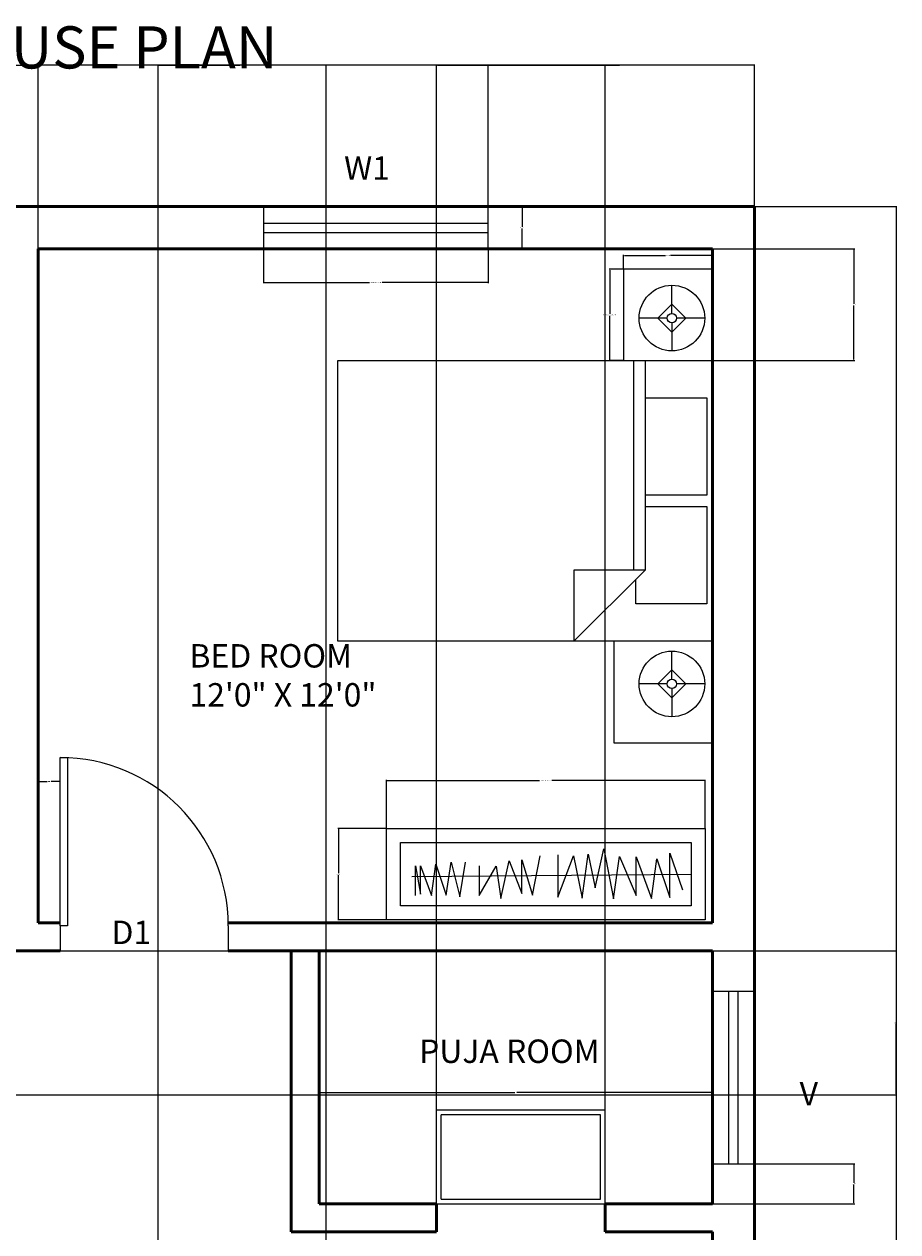
# Model space of a CAD drawing. Units: inches. Extents: x 437 to 811, y 2074 to 2699.
# Tile 4 of 4: x 624 to 811, y 2441 to 2699. Entities that reach past the tile are written whole.
import ezdxf

# ---------------------------------------------------------------- set-up
doc = ezdxf.new("R2010")
doc.units = ezdxf.units.IN
for name, color, linetype, lineweight in [('A-ANNO-DIMS', 2, 'Continuous', 18), ('A-ANNO-TEXT', 7, 'Continuous', 18), ('A-ANNO-TTLB', 7, 'Continuous', 35), ('A-AREA-IDEN', 7, 'Continuous', 25), ('A-DOOR', 4, 'Continuous', 25), ('A-FLOR-CASE', 9, 'Continuous', 25), ('A-FURN', 8, 'Continuous', 18), ('A-GLAZ', 4, 'Continuous', 18), ('A-WALL', 7, 'Continuous', 50)]:
    doc.layers.add(name, color=color, linetype=linetype, lineweight=lineweight)
doc.styles.get("Standard").update_dxf_attribs({"font": 'arial.ttf'})
doc.dimstyles.get("Standard").update_dxf_attribs({"dimtxt": 0.18, "dimasz": 0.18, "dimexe": 0.18, "dimexo": 0.0625, "dimgap": 0.09, "dimtad": 0, "dimtih": 1, "dimtoh": 1, "dimdec": 4, "dimzin": 0, "dimdsep": 46, "dimtxsty": 'Standard', "dimcen": 0.09, "dimadec": 0, "dimazin": 0, "dimtfac": 1, "dimtdec": 4, "dimtofl": 0, "dimtmove": 0, "dimatfit": 3, "dimfxl": 1, "dimtolj": 1, "dimtzin": 0, "dimarcsym": 0})

# ---------------------------------------------------------------- blocks, each defined once
blk = doc.blocks.new('Bed - Queen')
for p, q in [((0, -80.00003), (0, 0)), ((0, 0), (59.99999, 0)), ((59.99999, 0), (59.99999, -80.00003)), ((7.99999, -1.2), (28.79998, -1.2)), ((7.99999, -14.4), (7.99999, -1.2)), ((28.79998, -1.2), (28.79998, -14.4)), ((31.19999, -1.2), (51.99999, -1.2)), ((31.19999, -14.4), (31.19999, -1.2)), ((51.99999, -1.2), (51.99999, -16.4)), ((0, -14.4), (44.8, -14.4)), ((59.99999, -29.6), (44.8, -14.4)), ((44.8, -14.4), (44.8, -29.6)), ((44.8, -16.8), (0, -16.8)), ((51.99999, -16.4), (46.79936, -16.4)), ((44.8, -29.6), (59.99999, -29.6)), ((59.99999, -80.00003), (0, -80.00003))]:
    blk.add_line(p, q)
blk = doc.blocks.new('Lamp - Table')
for p, q in [((0, 7), (0, 1)), ((0, 3), (-3, 0)), ((3, 0), (0, 3)), ((-1, 0), (-7, 0)), ((-3, 0), (0, -3)), ((0, -3), (3, 0)), ((1, 0), (7, 0)), ((0, -1), (0, -7))]:
    blk.add_line(p, q)
for radius in [7, 1]:
    blk.add_circle((0, 0), radius)
blk = doc.blocks.new('*U10')
for p, q in [((0, 0), (0, -6)), ((40, 0), (40, -6))]:
    blk.add_line(p, q)
blk.add_lwpolyline([(0, 0), (0, 40), (1.75, 40), (1.75, 0)], close=True)
blk.add_arc((0, 0), 40, 0, 90)
blk = doc.blocks.new('WIN-W1-48IN')
for p, q in [((0, 5.5), (48, 5.5)), ((0, 3.5), (48, 3.5))]:
    blk.add_line(p, q)
blk.add_lwpolyline([(0, 0), (48, 0), (48, 9), (0, 9)], close=True)
blk = doc.blocks.new('VENT-V')
for p, q in [((9, 36.83), (0, 36.83)), ((0, 36.83), (0, 0)), ((3.5, 0), (3.5, 36.83)), ((5.5, 0), (5.5, 36.83)), ((9, 0), (9, 36.83)), ((0, 0), (9, 0))]:
    blk.add_line(p, q)
blk = doc.blocks.new('WARDROBE-BEDROOM')
for p, q in [((31.2, 5.25), (32.85, 13.72)), ((36.63, 13.91), (36.63, 4.86)), ((36.63, 4.86), (39.94, 13.72)), ((39.94, 13.72), (41.79, 4.67)), ((41.79, 4.67), (43.13, 14.04)), ((43.13, 14.04), (44.6, 6.84)), ((44.6, 6.84), (46.44, 15.19)), ((46.44, 15.19), (48.48, 4.48)), ((48.48, 4.48), (49.82, 13.53)), ((49.82, 13.53), (53.33, 5.18)), ((53.33, 5.18), (53.33, 13.47)), ((53.33, 13.47), (56.64, 4.54)), ((56.64, 4.54), (57.73, 13.02)), ((57.73, 13.02), (60.53, 4.8)), ((60.53, 4.8), (60.53, 14.29)), ((60.53, 14.29), (63.21, 6.39)), ((6.24, 5.24), (6.24, 11.53)), ((6.24, 11.53), (7.31, 5.48)), ((7.31, 5.48), (7.31, 11.54)), ((7.31, 11.54), (9.63, 5.2)), ((9.63, 5.2), (10.54, 11.9)), ((10.54, 11.9), (12.78, 5.28)), ((12.78, 5.28), (13.81, 12.34)), ((13.81, 12.34), (15.69, 4.96)), ((15.69, 4.96), (16.88, 12.37)), ((19.79, 11.56), (19.79, 5.18)), ((19.79, 5.18), (23.42, 11.48)), ((23.42, 11.48), (24.44, 4.55)), ((24.44, 4.55), (26.22, 12.64)), ((26.22, 12.64), (28.9, 5.63)), ((28.9, 5.63), (28.9, 12.83)), ((28.9, 12.83), (31.2, 5.25)), ((5.43, 9.27), (65.08, 9.77))]:
    blk.add_line(p, q)
for points in [[(0, 19.54), (68.08, 19.54), (68.08, 0), (0, 0)], [(3, 16.54), (65.08, 16.54), (65.08, 3), (3, 3)]]:
    blk.add_lwpolyline(points, close=True)
blk = doc.blocks.new('NIGHTSTAND-SMALL')
for p, q in [((0, 19.48), (0, 0)), ((19, 0), (19, 19.48)), ((0, 0), (19, 0))]:
    blk.add_line(p, q)
blk = doc.blocks.new('NIGHTSTAND-LARGE')
for p, q in [((0, 0), (0, 21.74)), ((0, 21.74), (21.02, 21.74)), ((21.02, 21.74), (21.02, 0))]:
    blk.add_line(p, q)
blk = doc.blocks.new('*D18')
at = {"layer": 'A-ANNO-DIMS', "color": 0, "lineweight": -2, "transparency": 16777216}
for p, q in [((675.12, 2650.74), (675.12, 2643.42)), ((723.12, 2650.74), (723.12, 2643.42)), ((675.3, 2643.6), (697.77, 2643.6)), ((722.94, 2643.6), (700.46, 2643.6))]:
    blk.add_line(p, q, dxfattribs=at)
at = {"layer": 'A-ANNO-DIMS', "color": 0, "transparency": 16777216}
for points in [[(675.3, 2643.63), (675.3, 2643.57), (675.12, 2643.6)], [(722.94, 2643.63), (722.94, 2643.57), (723.12, 2643.6)]]:
    blk.add_solid(points, dxfattribs=at)
at = {"layer": 'Defpoints', "color": 0, "transparency": 16777216}
for p in [(675.12, 2650.8), (723.12, 2650.8), (723.12, 2643.6)]:
    blk.add_point(p, dxfattribs=at)
at = {"layer": 'A-ANNO-DIMS', "color": 0, "transparency": 16777216, "insert": (699.12, 2643.6), "char_height": 0.18, "attachment_point": 5}
blk.add_mtext('\\A1;W1 WINDOW 48 TYP.', dxfattribs=at)
blk = doc.blocks.new('*D19')
at = {"layer": 'A-ANNO-DIMS', "color": 0, "lineweight": -2, "transparency": 16777216}
for p, q in [((723.18, 2659.8), (730.5, 2659.8)), ((730.32, 2659.62), (730.32, 2655.48)), ((730.32, 2650.98), (730.32, 2655.12)), ((723.18, 2650.8), (730.5, 2650.8))]:
    blk.add_line(p, q, dxfattribs=at)
at = {"layer": 'A-ANNO-DIMS', "color": 0, "transparency": 16777216}
for points in [[(730.29, 2659.62), (730.35, 2659.62), (730.32, 2659.8)], [(730.29, 2650.98), (730.35, 2650.98), (730.32, 2650.8)]]:
    blk.add_solid(points, dxfattribs=at)
at = {"layer": 'Defpoints', "color": 0, "transparency": 16777216}
for p in [(723.12, 2659.8), (730.32, 2659.8), (723.12, 2650.8)]:
    blk.add_point(p, dxfattribs=at)
at = {"layer": 'A-ANNO-DIMS', "color": 0, "transparency": 16777216, "insert": (730.32, 2655.3), "char_height": 0.18, "attachment_point": 5}
blk.add_mtext('\\A1;9 TYP.', dxfattribs=at)
blk = doc.blocks.new('*D22')
at = {"layer": 'A-ANNO-DIMS', "color": 0, "lineweight": -2, "transparency": 16777216}
for p, q in [((751.94, 2646.43), (748.91, 2646.43)), ((749.09, 2646.25), (749.09, 2636.89)), ((749.09, 2627.13), (749.09, 2636.48)), ((751.94, 2626.95), (748.91, 2626.95))]:
    blk.add_line(p, q, dxfattribs=at)
at = {"layer": 'A-ANNO-DIMS', "color": 0, "transparency": 16777216}
for points in [[(749.06, 2646.25), (749.12, 2646.25), (749.09, 2646.43)], [(749.06, 2627.13), (749.12, 2627.13), (749.09, 2626.95)]]:
    blk.add_solid(points, dxfattribs=at)
at = {"layer": 'Defpoints', "color": 0, "transparency": 16777216}
for p in [(752.01, 2646.43), (749.09, 2626.95), (752.01, 2626.95)]:
    blk.add_point(p, dxfattribs=at)
at = {"layer": 'A-ANNO-DIMS', "color": 0, "transparency": 16777216, "insert": (749.09, 2636.69), "char_height": 0.18, "attachment_point": 5}
blk.add_mtext('\\A1;NIGHTSTAND (S) 19 TYP.', dxfattribs=at)
blk = doc.blocks.new('*D23')
at = {"layer": 'A-ANNO-DIMS', "color": 0, "lineweight": -2, "transparency": 16777216}
for p, q in [((752.01, 2646.49), (752.01, 2649.53)), ((771, 2646.49), (771, 2649.53)), ((752.19, 2649.35), (760.99, 2649.35)), ((770.82, 2649.35), (762.03, 2649.35))]:
    blk.add_line(p, q, dxfattribs=at)
at = {"layer": 'A-ANNO-DIMS', "color": 0, "transparency": 16777216}
for points in [[(752.19, 2649.38), (752.19, 2649.32), (752.01, 2649.35)], [(770.82, 2649.38), (770.82, 2649.32), (771, 2649.35)]]:
    blk.add_solid(points, dxfattribs=at)
at = {"layer": 'Defpoints', "color": 0, "transparency": 16777216}
for p in [(752.01, 2649.35), (752.01, 2646.43), (771, 2646.43)]:
    blk.add_point(p, dxfattribs=at)
at = {"layer": 'A-ANNO-DIMS', "color": 0, "transparency": 16777216, "insert": (761.51, 2649.35), "char_height": 0.18, "attachment_point": 5}
blk.add_mtext('\\A1;19 TYP.', dxfattribs=at)
blk = doc.blocks.new('*D30')
at = {"layer": 'A-ANNO-DIMS', "color": 0, "lineweight": -2, "transparency": 16777216}
for p, q in [((701.35, 2527.04), (701.35, 2537.37)), ((701.53, 2537.19), (734.09, 2537.19)), ((769.25, 2537.19), (736.7, 2537.19)), ((769.43, 2527.04), (769.43, 2537.37))]:
    blk.add_line(p, q, dxfattribs=at)
at = {"layer": 'A-ANNO-DIMS', "color": 0, "transparency": 16777216}
for points in [[(701.53, 2537.22), (701.53, 2537.16), (701.35, 2537.19)], [(769.25, 2537.22), (769.25, 2537.16), (769.43, 2537.19)]]:
    blk.add_solid(points, dxfattribs=at)
at = {"layer": 'Defpoints', "color": 0, "transparency": 16777216}
for p in [(769.43, 2537.19), (701.35, 2526.98), (769.43, 2526.98)]:
    blk.add_point(p, dxfattribs=at)
at = {"layer": 'A-ANNO-DIMS', "color": 0, "transparency": 16777216, "insert": (735.39, 2537.19), "char_height": 0.18, "attachment_point": 5}
blk.add_mtext('\\A1;WARDROBE 68 TYP.', dxfattribs=at)
blk = doc.blocks.new('*D31')
at = {"layer": 'A-ANNO-DIMS', "color": 0, "lineweight": -2, "transparency": 16777216}
for p, q in [((701.29, 2526.98), (690.96, 2526.98)), ((691.14, 2526.8), (691.14, 2517.39)), ((691.14, 2507.61), (691.14, 2517.02)), ((701.29, 2507.43), (690.96, 2507.43))]:
    blk.add_line(p, q, dxfattribs=at)
at = {"layer": 'A-ANNO-DIMS', "color": 0, "transparency": 16777216}
for points in [[(691.11, 2526.8), (691.17, 2526.8), (691.14, 2526.98)], [(691.11, 2507.61), (691.17, 2507.61), (691.14, 2507.43)]]:
    blk.add_solid(points, dxfattribs=at)
at = {"layer": 'Defpoints', "color": 0, "transparency": 16777216}
for p in [(691.14, 2526.98), (701.35, 2526.98), (701.35, 2507.43)]:
    blk.add_point(p, dxfattribs=at)
at = {"layer": 'A-ANNO-DIMS', "color": 0, "transparency": 16777216, "insert": (691.14, 2517.21), "char_height": 0.18, "attachment_point": 5}
blk.add_mtext('\\A1;20 TYP.', dxfattribs=at)
blk = doc.blocks.new('*D45')
at = {"layer": 'A-ANNO-DIMS', "color": 0, "lineweight": -2, "transparency": 16777216}
for p, q in [((652.6, 2128.86), (652.6, 2690.18)), ((652.78, 2690), (670.09, 2690)), ((688.34, 2690), (671.02, 2690)), ((688.52, 2128.86), (688.52, 2690.18))]:
    blk.add_line(p, q, dxfattribs=at)
at = {"layer": 'A-ANNO-DIMS', "color": 0, "transparency": 16777216}
for points in [[(652.78, 2690.03), (652.78, 2689.97), (652.6, 2690)], [(688.34, 2690.03), (688.34, 2689.97), (688.52, 2690)]]:
    blk.add_solid(points, dxfattribs=at)
at = {"layer": 'Defpoints', "color": 0, "transparency": 16777216}
for p in [(688.52, 2690), (652.6, 2128.8), (688.52, 2128.8)]:
    blk.add_point(p, dxfattribs=at)
at = {"layer": 'A-ANNO-DIMS', "color": 0, "transparency": 16777216, "insert": (670.56, 2690), "char_height": 0.18, "attachment_point": 5}
blk.add_mtext('\\A1;35.924', dxfattribs=at)
blk = doc.blocks.new('*D49')
at = {"layer": 'A-ANNO-DIMS', "color": 0, "lineweight": -2, "transparency": 16777216}
for p, q in [((723.12, 2659.86), (723.12, 2690.18)), ((723.3, 2690), (751.17, 2690)), ((779.82, 2690), (751.95, 2690)), ((780, 2659.86), (780, 2690.18))]:
    blk.add_line(p, q, dxfattribs=at)
at = {"layer": 'A-ANNO-DIMS', "color": 0, "transparency": 16777216}
for points in [[(723.3, 2690.03), (723.3, 2689.97), (723.12, 2690)], [(779.82, 2690.03), (779.82, 2689.97), (780, 2690)]]:
    blk.add_solid(points, dxfattribs=at)
at = {"layer": 'Defpoints', "color": 0, "transparency": 16777216}
for p in [(780, 2690), (723.12, 2659.8), (780, 2659.8)]:
    blk.add_point(p, dxfattribs=at)
at = {"layer": 'A-ANNO-DIMS', "color": 0, "transparency": 16777216, "insert": (751.56, 2690), "char_height": 0.18, "attachment_point": 5}
blk.add_mtext('\\A1;56.89', dxfattribs=at)
blk = doc.blocks.new('*D50')
at = {"layer": 'A-ANNO-DIMS', "color": 0, "lineweight": -2, "transparency": 16777216}
for p, q in [((621, 2650.86), (621, 2690.18)), ((621.18, 2690), (623.86, 2690)), ((626.82, 2690), (624.15, 2690)), ((627, 2650.86), (627, 2690.18))]:
    blk.add_line(p, q, dxfattribs=at)
at = {"layer": 'A-ANNO-DIMS', "color": 0, "transparency": 16777216}
for points in [[(621.18, 2690.03), (621.18, 2689.97), (621, 2690)], [(626.82, 2690.03), (626.82, 2689.97), (627, 2690)]]:
    blk.add_solid(points, dxfattribs=at)
at = {"layer": 'Defpoints', "color": 0, "transparency": 16777216}
for p in [(627, 2690), (621, 2650.8), (627, 2650.8)]:
    blk.add_point(p, dxfattribs=at)
at = {"layer": 'A-ANNO-DIMS', "color": 0, "transparency": 16777216, "insert": (624, 2690), "char_height": 0.18, "attachment_point": 5}
blk.add_mtext('\\A1;6', dxfattribs=at)
blk = doc.blocks.new('*D56')
at = {"layer": 'A-ANNO-DIMS', "color": 0, "lineweight": -2, "transparency": 16777216}
for p, q in [((771.07, 2455.34), (801.38, 2455.34)), ((801.2, 2455.16), (801.2, 2451.25)), ((801.2, 2446.98), (801.2, 2450.89)), ((771.07, 2446.8), (801.38, 2446.8))]:
    blk.add_line(p, q, dxfattribs=at)
at = {"layer": 'A-ANNO-DIMS', "color": 0, "transparency": 16777216}
for points in [[(801.17, 2455.16), (801.23, 2455.16), (801.2, 2455.34)], [(801.17, 2446.98), (801.23, 2446.98), (801.2, 2446.8)]]:
    blk.add_solid(points, dxfattribs=at)
at = {"layer": 'Defpoints', "color": 0, "transparency": 16777216}
for p in [(771, 2455.34), (771, 2446.8), (801.2, 2446.8)]:
    blk.add_point(p, dxfattribs=at)
at = {"layer": 'A-ANNO-DIMS', "color": 0, "transparency": 16777216, "insert": (801.2, 2451.07), "char_height": 0.18, "attachment_point": 5}
blk.add_mtext('\\A1;8.538', dxfattribs=at)
blk = doc.blocks.new('*D59')
at = {"layer": 'A-ANNO-DIMS', "color": 0, "lineweight": -2, "transparency": 16777216}
for p, q in [((567.07, 2500.8), (810.38, 2500.8)), ((810.2, 2500.62), (810.2, 2485.62)), ((810.2, 2470.27), (810.2, 2485.26)), ((567.07, 2470.09), (810.38, 2470.09))]:
    blk.add_line(p, q, dxfattribs=at)
at = {"layer": 'A-ANNO-DIMS', "color": 0, "transparency": 16777216}
for points in [[(810.17, 2500.62), (810.23, 2500.62), (810.2, 2500.8)], [(810.17, 2470.27), (810.23, 2470.27), (810.2, 2470.09)]]:
    blk.add_solid(points, dxfattribs=at)
at = {"layer": 'Defpoints', "color": 0, "transparency": 16777216}
for p in [(567, 2500.8), (810.2, 2500.8), (567, 2470.09)]:
    blk.add_point(p, dxfattribs=at)
at = {"layer": 'A-ANNO-DIMS', "color": 0, "transparency": 16777216, "insert": (810.2, 2485.44), "char_height": 0.18, "attachment_point": 5}
blk.add_mtext('\\A1;30.714', dxfattribs=at)
blk = doc.blocks.new('*D60')
at = {"layer": 'A-ANNO-DIMS', "color": 0, "lineweight": -2, "transparency": 16777216}
for p, q in [((687, 2500.74), (687, 2470.42)), ((771, 2500.74), (771, 2470.42)), ((687.18, 2470.6), (728.79, 2470.6)), ((770.82, 2470.6), (729.22, 2470.6))]:
    blk.add_line(p, q, dxfattribs=at)
at = {"layer": 'A-ANNO-DIMS', "color": 0, "transparency": 16777216}
for points in [[(687.18, 2470.63), (687.18, 2470.57), (687, 2470.6)], [(770.82, 2470.63), (770.82, 2470.57), (771, 2470.6)]]:
    blk.add_solid(points, dxfattribs=at)
at = {"layer": 'Defpoints', "color": 0, "transparency": 16777216}
for p in [(687, 2500.8), (771, 2500.8), (687, 2470.6)]:
    blk.add_point(p, dxfattribs=at)
at = {"layer": 'A-ANNO-DIMS', "color": 0, "transparency": 16777216, "insert": (729, 2470.6), "char_height": 0.18, "attachment_point": 5}
blk.add_mtext('\\A1;84', dxfattribs=at)
blk = doc.blocks.new('*D76')
at = {"layer": 'A-ANNO-DIMS', "color": 0, "lineweight": -2, "transparency": 16777216}
for p, q in [((627, 2506.86), (627, 2537.18)), ((627.18, 2537), (628.94, 2537)), ((631.49, 2537), (629.74, 2537)), ((631.67, 2506.86), (631.67, 2537.18))]:
    blk.add_line(p, q, dxfattribs=at)
at = {"layer": 'A-ANNO-DIMS', "color": 0, "transparency": 16777216}
for points in [[(627.18, 2537.03), (627.18, 2536.97), (627, 2537)], [(631.49, 2537.03), (631.49, 2536.97), (631.67, 2537)]]:
    blk.add_solid(points, dxfattribs=at)
at = {"layer": 'Defpoints', "color": 0, "transparency": 16777216}
for p in [(631.67, 2537), (627, 2506.8), (631.67, 2506.8)]:
    blk.add_point(p, dxfattribs=at)
at = {"layer": 'A-ANNO-DIMS', "color": 0, "transparency": 16777216, "insert": (629.34, 2537), "char_height": 0.18, "attachment_point": 5}
blk.add_mtext('\\A1;4.665', dxfattribs=at)
blk = doc.blocks.new('*D77')
at = {"layer": 'A-ANNO-DIMS', "color": 0, "lineweight": -2, "transparency": 16777216}
for p, q in [((712.06, 2466.89), (712.06, 2690.18)), ((712.24, 2690), (729.84, 2690)), ((747.88, 2690), (730.28, 2690)), ((748.06, 2466.89), (748.06, 2690.18))]:
    blk.add_line(p, q, dxfattribs=at)
at = {"layer": 'A-ANNO-DIMS', "color": 0, "transparency": 16777216}
for points in [[(712.24, 2690.03), (712.24, 2689.97), (712.06, 2690)], [(747.88, 2690.03), (747.88, 2689.97), (748.06, 2690)]]:
    blk.add_solid(points, dxfattribs=at)
at = {"layer": 'Defpoints', "color": 0, "transparency": 16777216}
for p in [(748.06, 2690), (712.06, 2466.82), (748.06, 2466.82)]:
    blk.add_point(p, dxfattribs=at)
at = {"layer": 'A-ANNO-DIMS', "color": 0, "transparency": 16777216, "insert": (730.06, 2690), "char_height": 0.18, "attachment_point": 5}
blk.add_mtext('\\A1;36', dxfattribs=at)
blk = doc.blocks.new('*D80')
at = {"layer": 'A-ANNO-DIMS', "color": 0, "lineweight": -2, "transparency": 16777216}
for p, q in [((771.07, 2650.8), (801.38, 2650.8)), ((801.2, 2650.62), (801.2, 2639.05)), ((801.2, 2627.13), (801.2, 2638.69)), ((771.07, 2626.95), (801.38, 2626.95))]:
    blk.add_line(p, q, dxfattribs=at)
at = {"layer": 'A-ANNO-DIMS', "color": 0, "transparency": 16777216}
for points in [[(801.17, 2650.62), (801.23, 2650.62), (801.2, 2650.8)], [(801.17, 2627.13), (801.23, 2627.13), (801.2, 2626.95)]]:
    blk.add_solid(points, dxfattribs=at)
at = {"layer": 'Defpoints', "color": 0, "transparency": 16777216}
for p in [(771, 2650.8), (771, 2626.95), (801.2, 2626.95)]:
    blk.add_point(p, dxfattribs=at)
at = {"layer": 'A-ANNO-DIMS', "color": 0, "transparency": 16777216, "insert": (801.2, 2638.87), "char_height": 0.18, "attachment_point": 5}
blk.add_mtext('\\A1;23.854', dxfattribs=at)
blk = doc.blocks.new('*D86')
at = {"layer": 'A-ANNO-DIMS', "color": 0, "lineweight": -2, "transparency": 16777216}
for p, q in [((468, 2659.86), (468, 2690.18)), ((468.18, 2690), (623.72, 2690)), ((779.82, 2690), (624.29, 2690)), ((780, 2659.86), (780, 2690.18))]:
    blk.add_line(p, q, dxfattribs=at)
at = {"layer": 'A-ANNO-DIMS', "color": 0, "transparency": 16777216}
for points in [[(468.18, 2690.03), (468.18, 2689.97), (468, 2690)], [(779.82, 2690.03), (779.82, 2689.97), (780, 2690)]]:
    blk.add_solid(points, dxfattribs=at)
at = {"layer": 'Defpoints', "color": 0, "transparency": 16777216}
for p in [(780, 2690), (468, 2659.8), (780, 2659.8)]:
    blk.add_point(p, dxfattribs=at)
at = {"layer": 'A-ANNO-DIMS', "color": 0, "transparency": 16777216, "insert": (624, 2690), "char_height": 0.18, "attachment_point": 5}
blk.add_mtext('\\A1;312', dxfattribs=at)
blk = doc.blocks.new('*D87')
at = {"layer": 'A-ANNO-DIMS', "color": 0, "lineweight": -2, "transparency": 16777216}
for p, q in [((780.07, 2659.8), (810.38, 2659.8)), ((810.2, 2659.62), (810.2, 2382.48)), ((810.2, 2104.98), (810.2, 2382.12)), ((698.21, 2104.8), (810.38, 2104.8))]:
    blk.add_line(p, q, dxfattribs=at)
at = {"layer": 'A-ANNO-DIMS', "color": 0, "transparency": 16777216}
for points in [[(810.17, 2659.62), (810.23, 2659.62), (810.2, 2659.8)], [(810.17, 2104.98), (810.23, 2104.98), (810.2, 2104.8)]]:
    blk.add_solid(points, dxfattribs=at)
at = {"layer": 'Defpoints', "color": 0, "transparency": 16777216}
for p in [(780, 2659.8), (810.2, 2659.8), (698.15, 2104.8)]:
    blk.add_point(p, dxfattribs=at)
at = {"layer": 'A-ANNO-DIMS', "color": 0, "transparency": 16777216, "insert": (810.2, 2382.3), "char_height": 0.18, "attachment_point": 5}
blk.add_mtext('\\A1;555', dxfattribs=at)

msp = doc.modelspace()

# ---------------------------------------------------------------- linework, layer by layer
at = {"layer": 'A-FLOR-CASE'}
for p, q in [((748.0584, 2466.8236), (712.0584, 2466.8236)), ((712.0584, 2446.7995), (712.0584, 2466.8236)), ((748.0584, 2446.7995), (748.0584, 2466.8236)), ((713.0584, 2447.7995), (713.0584, 2465.8236)), ((747.0584, 2465.8236), (713.0584, 2465.8236)), ((747.0584, 2447.7995), (747.0584, 2465.8236)), ((712.0584, 2446.7995), (748.0584, 2446.7995)), ((713.0584, 2447.7995), (747.0584, 2447.7995))]:
    msp.add_line(p, q, dxfattribs=at)
at = {"layer": 'A-WALL'}
for p, q in [((780.0049, 2659.7995), (468.0049, 2659.7995)), ((780.0049, 2206.7995), (780.0049, 2659.7995)), ((627.0049, 2506.7995), (627.0049, 2650.7995)), ((627.0049, 2650.7995), (771.0049, 2650.7995)), ((771.0049, 2506.7995), (771.0049, 2650.7995)), ((627.0049, 2506.7995), (631.6694, 2506.7995)), ((667.5883, 2506.7995), (771.0049, 2506.7995)), ((617.0035, 2500.7995), (631.6694, 2500.7995)), ((667.5935, 2500.7995), (771.0049, 2500.7995)), ((681.0049, 2440.7995), (681.0049, 2500.7995)), ((687.0049, 2446.7995), (687.0049, 2500.7995)), ((771.0049, 2500.7995), (771.0049, 2446.7995)), ((712.0584, 2446.7995), (687.0049, 2446.7995)), ((712.0584, 2446.7995), (712.0584, 2440.7995)), ((771.0049, 2446.7995), (748.0584, 2446.7995)), ((748.0584, 2446.7995), (748.0584, 2440.7995)), ((712.0584, 2440.7995), (681.0049, 2440.7995)), ((771.0049, 2440.7995), (748.0584, 2440.7995)), ((771.0049, 2440.7995), (771.0049, 2206.7995))]:
    msp.add_line(p, q, dxfattribs=at)

# ---------------------------------------------------------------- block references
at = {"layer": 'A-DOOR', "xscale": 0.8981017077080947, "yscale": 0.8981017077080947, "zscale": 0.8981017077080947}
msp.add_blockref('*U10', (631.6694, 2506.1881), dxfattribs=at)
at = {"layer": 'A-FURN'}
for name, p, rotation in [('NIGHTSTAND-SMALL', (771.0048, 2646.427), 180), ('Lamp - Table', (762.3331, 2635.9901), 270), ('Bed - Queen', (771.0049, 2626.9454), 270), ('NIGHTSTAND-LARGE', (771.0048, 2566.945), 180), ('Lamp - Table', (762.3331, 2557.8458), 270)]:
    msp.add_blockref(name, p, dxfattribs=dict(at, rotation=rotation))
msp.add_blockref('WARDROBE-BEDROOM', (701.3499, 2507.434), dxfattribs=at)
at = {"layer": 'A-GLAZ'}
for name, p in [('WIN-W1-48IN', (675.1155, 2650.799)), ('VENT-V', (771.005, 2455.3372))]:
    msp.add_blockref(name, p, dxfattribs=at)

# ---------------------------------------------------------------- texts
at = {"layer": 'A-ANNO-TEXT', "char_height": 5, "width": 52.048983, "attachment_point": 1}
for s, insert in [('W1', (692.3327, 2670.5384)), ('D1', (642.6541, 2507.2721)), ('V', (789.6068, 2472.8152))]:
    msp.add_mtext(s, dxfattribs=dict(at, insert=insert))
at = {"layer": 'A-ANNO-TTLB', "insert": (553.7348, 2698.3139), "char_height": 9, "width": 177.859247, "attachment_point": 1}
msp.add_mtext("25' X 42' HOUSE PLAN", dxfattribs=at)
at = {"layer": 'A-AREA-IDEN', "char_height": 5, "width": 52.048983, "attachment_point": 1}
for s, insert in [('BED ROOM\\P12\'0" X 12\'0"', (659.3048, 2566.3477)), ('PUJA ROOM', (708.345, 2481.8812))]:
    msp.add_mtext(s, dxfattribs=dict(at, insert=insert))

# ---------------------------------------------------------------- dimensions: what is measured, and where the dimension line sits
at = {"layer": 'A-ANNO-DIMS'}
for base, p1, p2, override, picture, middle in [((780.0049, 2689.9995), (468.0049, 2659.7995), (780.0049, 2659.7995), {"dimdec": 0, "dimlfac": 1, "dimrnd": 0, "dimzin": 0, "dimdsep": 46, "dimlunit": 2}, '*D86', (624.0049, 2689.9995)), ((627.0049, 2689.9995), (621.0049, 2650.7995), (627.0049, 2650.7995), {"dimdec": 0, "dimlfac": 1, "dimrnd": 0, "dimzin": 0, "dimdsep": 46, "dimlunit": 2}, '*D50', (624.0049, 2689.9995)), ((688.5196, 2689.9995), (652.5955, 2128.7995), (688.5196, 2128.7995), {"dimdec": 3, "dimlfac": 1, "dimrnd": 0, "dimzin": 0, "dimdsep": 46, "dimlunit": 2}, '*D45', (670.5576, 2689.9995)), ((748.0584, 2689.9995), (712.0584, 2466.8236), (748.0584, 2466.8236), {"dimdec": 0, "dimlfac": 1, "dimrnd": 0, "dimzin": 0, "dimdsep": 46, "dimlunit": 2}, '*D77', (730.0584, 2689.9995)), ((780.0049, 2689.9995), (723.1152, 2659.7995), (780.0049, 2659.7995), {"dimdec": 2, "dimlfac": 1, "dimrnd": 0, "dimzin": 0, "dimdsep": 46, "dimlunit": 2}, '*D49', (751.56, 2689.9995)), ((631.66943, 2536.99945), (627.00488, 2506.79945), (631.66943, 2506.79945), {"dimdec": 3, "dimlfac": 1, "dimrnd": 0, "dimzin": 0, "dimdsep": 46, "dimlunit": 2}, '*D76', (629.33716, 2536.99945))]:
    dim = msp.add_linear_dim(base=base, p1=p1, p2=p2, dimstyle='Standard', override=override, dxfattribs=at)
    dim.commit()
    dim.dimension.update_dxf_attribs({"geometry": picture, "text_midpoint": middle})
for base, p1, p2, angle, override, picture, middle in [((810.2049, 2659.7995), (698.148, 2104.7995), (780.0049, 2659.7995), 90, {"dimdec": 0, "dimlfac": 1, "dimrnd": 0, "dimzin": 0, "dimdsep": 46, "dimlunit": 2}, '*D87', (810.2049, 2382.2995)), ((801.2049, 2626.9454), (771.0049, 2650.7995), (771.0049, 2626.9454), 270, {"dimdec": 3, "dimlfac": 1, "dimrnd": 0, "dimzin": 0, "dimdsep": 46, "dimlunit": 2}, '*D80', (801.2049, 2638.8724)), ((810.2049, 2500.7995), (567.0049, 2470.0858), (567.0049, 2500.7995), 90, {"dimdec": 3, "dimlfac": 1, "dimrnd": 0, "dimzin": 0, "dimdsep": 46, "dimlunit": 2}, '*D59', (810.2049, 2485.4426)), ((687.0049, 2470.5995), (771.0049, 2500.7995), (687.0049, 2500.7995), 180, {"dimdec": 0, "dimlfac": 1, "dimrnd": 0, "dimzin": 0, "dimdsep": 46, "dimlunit": 2}, '*D60', (729.0049, 2470.5995)), ((801.2049, 2446.7995), (771.0049, 2455.3375), (771.0049, 2446.7995), 270, {"dimdec": 3, "dimlfac": 1, "dimrnd": 0, "dimzin": 0, "dimdsep": 46, "dimlunit": 2}, '*D56', (801.2049, 2451.0685))]:
    dim = msp.add_linear_dim(base=base, p1=p1, p2=p2, angle=angle, dimstyle='Standard', override=override, dxfattribs=at)
    dim.commit()
    dim.dimension.update_dxf_attribs({"geometry": picture, "text_midpoint": middle})
for base, p1, p2, angle, text, picture, middle in [((730.3152, 2659.7995), (723.1152, 2650.7995), (723.1152, 2659.7995), 90, '<> TYP.', '*D19', (730.3152, 2655.2995)), ((752.0074, 2649.3495), (771.0049, 2646.4272), (752.0074, 2646.4272), 180, '<> TYP.', '*D23', (761.5061, 2649.3495)), ((749.0851, 2626.9454), (752.0074, 2646.4272), (752.0074, 2626.9454), 270, 'NIGHTSTAND (S) <> TYP.', '*D22', (749.0851, 2636.6863)), ((691.137, 2526.9769), (701.3498, 2507.4338), (701.3498, 2526.9769), 90, '<> TYP.', '*D31', (691.137, 2517.2054))]:
    dim = msp.add_linear_dim(base=base, p1=p1, p2=p2, angle=angle, text=text, dimstyle='Standard', override={"dimdec": 0, "dimlfac": 1, "dimrnd": 0, "dimzin": 0, "dimdsep": 46, "dimlunit": 2}, dxfattribs=at)
    dim.commit()
    dim.dimension.update_dxf_attribs({"geometry": picture, "text_midpoint": middle})
for base, p1, p2, text, picture, middle in [((723.1152, 2643.5995), (675.1152, 2650.7995), (723.1152, 2650.7995), 'W1 WINDOW <> TYP.', '*D18', (699.1152, 2643.5995)), ((769.4348, 2537.1896), (701.3498, 2526.9769), (769.4348, 2526.9769), 'WARDROBE <> TYP.', '*D30', (735.3923, 2537.1896))]:
    dim = msp.add_linear_dim(base=base, p1=p1, p2=p2, text=text, dimstyle='Standard', override={"dimdec": 0, "dimlfac": 1, "dimrnd": 0, "dimzin": 0, "dimdsep": 46, "dimlunit": 2}, dxfattribs=at)
    dim.commit()
    dim.dimension.update_dxf_attribs({"geometry": picture, "text_midpoint": middle})

doc.saveas('drawing.dxf')
